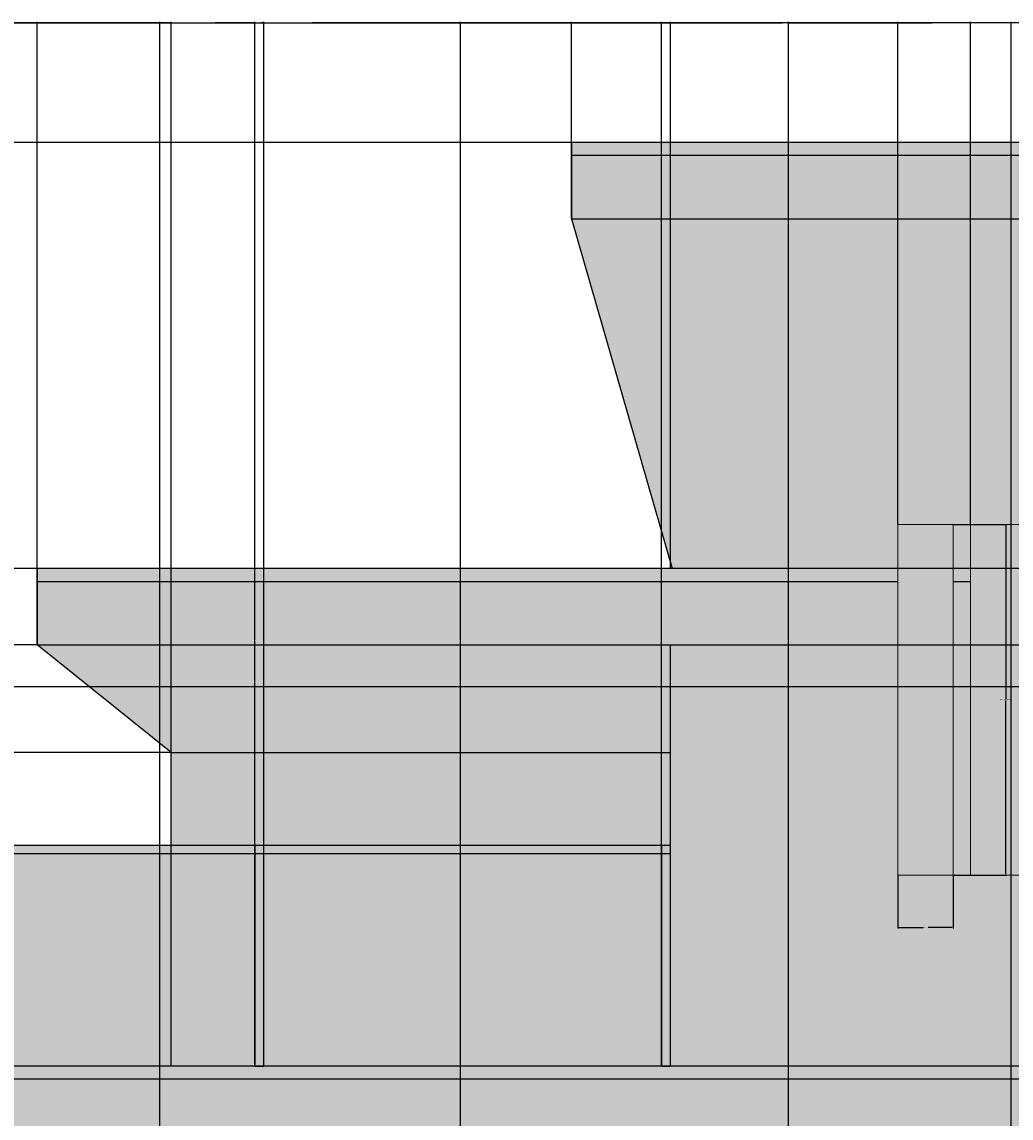
# Model space of a CAD drawing. Units: feet. Extents: x 2926 to 4178, y 965 to 1469.
# Tile 5 of 9: x 3040 to 3245, y 1241 to 1469. Entities that reach past the tile are written whole.
import ezdxf

# ---------------------------------------------------------------- set-up
doc = ezdxf.new("R2010")
doc.units = ezdxf.units.FT
for name, color, linetype, lineweight in [('A-ANNO-DIMS', 2, 'Continuous', 18), ('A-ELEV', 7, 'Continuous', 25), ('A-ELEV-DETL', 8, 'Continuous', 18), ('A-ELEV-PATT', 9, 'Continuous', 13)]:
    doc.layers.add(name, color=color, linetype=linetype, lineweight=lineweight)
doc.styles.get("Standard").update_dxf_attribs({"font": 'arial.ttf'})
doc.dimstyles.get("Standard").update_dxf_attribs({"dimtxt": 0.18, "dimasz": 0.18, "dimexe": 0.18, "dimexo": 0.0625, "dimgap": 0.09, "dimtad": 0, "dimtih": 1, "dimtoh": 1, "dimdec": 1, "dimzin": 0, "dimdsep": 46, "dimlunit": 3, "dimtxsty": 'Standard', "dimcen": 0.09, "dimadec": 0, "dimazin": 0, "dimtfac": 1, "dimtdec": 1, "dimtofl": 0, "dimtmove": 0, "dimatfit": 3, "dimfxl": 1, "dimtolj": 1, "dimtzin": 0, "dimarcsym": 0})

# ---------------------------------------------------------------- blocks, each defined once
blk = doc.blocks.new('FACADE-FIN')
blk.add_lwpolyline([(0, 72.66), (11.46, 72.66), (11.46, 0), (0, 0)], close=True)
blk.add_lwpolyline([(0, 72.66), (11.46, 72.66), (11.46, 0), (0, 0)], close=True)
blk = doc.blocks.new('*D4')
at = {"layer": 'A-ANNO-DIMS', "color": 0, "lineweight": -2, "transparency": 16777216}
for p, q in [((3232.87, 1364.4), (3243.89, 1364.4)), ((3243.71, 1364.22), (3243.71, 1328.25)), ((3243.71, 1291.91), (3243.71, 1327.88)), ((3232.87, 1291.73), (3243.89, 1291.73))]:
    blk.add_line(p, q, dxfattribs=at)
at = {"layer": 'A-ANNO-DIMS', "color": 0, "transparency": 16777216}
for points in [[(3243.68, 1364.22), (3243.74, 1364.22), (3243.71, 1364.4)], [(3243.68, 1291.91), (3243.74, 1291.91), (3243.71, 1291.73)]]:
    blk.add_solid(points, dxfattribs=at)
at = {"layer": 'Defpoints', "color": 0, "transparency": 16777216}
for p in [(3232.81, 1364.4), (3243.71, 1364.4), (3232.81, 1291.73)]:
    blk.add_point(p, dxfattribs=at)
at = {"layer": 'A-ANNO-DIMS', "color": 0, "transparency": 16777216, "insert": (3243.71, 1328.07), "char_height": 0.18, "attachment_point": 5}
blk.add_mtext('\\A1;FACADE FIN 73 TYP.', dxfattribs=at)
blk = doc.blocks.new('*D5')
at = {"layer": 'A-ANNO-DIMS', "color": 0, "lineweight": -2, "transparency": 16777216}
for p, q in [((3221.35, 1291.67), (3221.35, 1280.66)), ((3232.81, 1291.67), (3232.81, 1280.66)), ((3221.53, 1280.84), (3226.56, 1280.84)), ((3232.63, 1280.84), (3227.6, 1280.84))]:
    blk.add_line(p, q, dxfattribs=at)
at = {"layer": 'A-ANNO-DIMS', "color": 0, "transparency": 16777216}
for points in [[(3221.53, 1280.87), (3221.53, 1280.81), (3221.35, 1280.84)], [(3232.63, 1280.87), (3232.63, 1280.81), (3232.81, 1280.84)]]:
    blk.add_solid(points, dxfattribs=at)
at = {"layer": 'Defpoints', "color": 0, "transparency": 16777216}
for p in [(3221.35, 1291.73), (3232.81, 1291.73), (3232.81, 1280.84)]:
    blk.add_point(p, dxfattribs=at)
at = {"layer": 'A-ANNO-DIMS', "color": 0, "transparency": 16777216, "insert": (3227.08, 1280.84), "char_height": 0.18, "attachment_point": 5}
blk.add_mtext('\\A1;11 TYP.', dxfattribs=at)
blk = doc.blocks.new('*D10')
at = {"layer": 'A-ANNO-DIMS', "color": 0, "lineweight": -2, "transparency": 16777216}
for p, q in [((2952.4, 1298.4), (2952.4, 1468.62)), ((2952.58, 1468.44), (3195.09, 1468.44)), ((3438.39, 1468.44), (3195.88, 1468.44)), ((3438.57, 1443.71), (3438.57, 1468.62))]:
    blk.add_line(p, q, dxfattribs=at)
at = {"layer": 'A-ANNO-DIMS', "color": 0, "transparency": 16777216}
for points in [[(2952.58, 1468.47), (2952.58, 1468.41), (2952.4, 1468.44)], [(3438.39, 1468.47), (3438.39, 1468.41), (3438.57, 1468.44)]]:
    blk.add_solid(points, dxfattribs=at)
at = {"layer": 'Defpoints', "color": 0, "transparency": 16777216}
for p in [(3438.57, 1468.44), (3438.57, 1443.64), (2952.4, 1298.33)]:
    blk.add_point(p, dxfattribs=at)
at = {"layer": 'A-ANNO-DIMS', "color": 0, "transparency": 16777216, "insert": (3195.49, 1468.44), "char_height": 0.18, "attachment_point": 5}
blk.add_mtext('\\A1;486.2', dxfattribs=at)
blk = doc.blocks.new('*D17')
at = {"layer": 'A-ANNO-DIMS', "color": 0, "lineweight": -2, "transparency": 16777216}
for p, q in [((2952.34, 1252.14), (2926.57, 1252.14)), ((2926.75, 1251.96), (2926.75, 1235.86)), ((2926.75, 1219.4), (2926.75, 1235.5)), ((3198.58, 1219.22), (2926.57, 1219.22))]:
    blk.add_line(p, q, dxfattribs=at)
at = {"layer": 'A-ANNO-DIMS', "color": 0, "transparency": 16777216}
for points in [[(2926.72, 1251.96), (2926.78, 1251.96), (2926.75, 1252.14)], [(2926.72, 1219.4), (2926.78, 1219.4), (2926.75, 1219.22)]]:
    blk.add_solid(points, dxfattribs=at)
at = {"layer": 'Defpoints', "color": 0, "transparency": 16777216}
for p in [(2926.75, 1252.14), (2952.4, 1252.14), (3198.64, 1219.22)]:
    blk.add_point(p, dxfattribs=at)
at = {"layer": 'A-ANNO-DIMS', "color": 0, "transparency": 16777216, "insert": (2926.75, 1235.68), "char_height": 0.18, "attachment_point": 5}
blk.add_mtext('\\A1;32.92', dxfattribs=at)
blk = doc.blocks.new('*D19')
at = {"layer": 'A-ANNO-DIMS', "color": 0, "lineweight": -2, "transparency": 16777216}
for p, q in [((3335.85, 1330.74), (2926.57, 1330.74)), ((2926.75, 1330.56), (2926.75, 1314.5)), ((2926.75, 1298.08), (2926.75, 1314.14)), ((2952.34, 1297.9), (2926.57, 1297.9))]:
    blk.add_line(p, q, dxfattribs=at)
at = {"layer": 'A-ANNO-DIMS', "color": 0, "transparency": 16777216}
for points in [[(2926.72, 1330.56), (2926.78, 1330.56), (2926.75, 1330.74)], [(2926.72, 1298.08), (2926.78, 1298.08), (2926.75, 1297.9)]]:
    blk.add_solid(points, dxfattribs=at)
at = {"layer": 'Defpoints', "color": 0, "transparency": 16777216}
for p in [(2926.75, 1330.74), (3335.91, 1330.74), (2952.4, 1297.9)]:
    blk.add_point(p, dxfattribs=at)
at = {"layer": 'A-ANNO-DIMS', "color": 0, "transparency": 16777216, "insert": (2926.75, 1314.32), "char_height": 0.18, "attachment_point": 5}
blk.add_mtext('\\A1;32.85', dxfattribs=at)
blk = doc.blocks.new('*D20')
at = {"layer": 'A-ANNO-DIMS', "color": 0, "lineweight": -2, "transparency": 16777216}
for p, q in [((3042.86, 1355.28), (2926.57, 1355.28)), ((2926.75, 1355.1), (2926.75, 1343.19)), ((2926.75, 1330.92), (2926.75, 1342.83)), ((3335.85, 1330.74), (2926.57, 1330.74))]:
    blk.add_line(p, q, dxfattribs=at)
at = {"layer": 'A-ANNO-DIMS', "color": 0, "transparency": 16777216}
for points in [[(2926.72, 1355.1), (2926.78, 1355.1), (2926.75, 1355.28)], [(2926.72, 1330.92), (2926.78, 1330.92), (2926.75, 1330.74)]]:
    blk.add_solid(points, dxfattribs=at)
at = {"layer": 'Defpoints', "color": 0, "transparency": 16777216}
for p in [(2926.75, 1355.28), (3042.92, 1355.28), (3335.91, 1330.74)]:
    blk.add_point(p, dxfattribs=at)
at = {"layer": 'A-ANNO-DIMS', "color": 0, "transparency": 16777216, "insert": (2926.75, 1343.01), "char_height": 0.18, "attachment_point": 5}
blk.add_mtext('\\A1;24.533', dxfattribs=at)
blk = doc.blocks.new('*D21')
at = {"layer": 'A-ANNO-DIMS', "color": 0, "lineweight": -2, "transparency": 16777216}
for p, q in [((3153.63, 1443.64), (2926.57, 1443.64)), ((2926.75, 1443.46), (2926.75, 1399.64)), ((2926.75, 1355.46), (2926.75, 1399.28)), ((3042.86, 1355.28), (2926.57, 1355.28))]:
    blk.add_line(p, q, dxfattribs=at)
at = {"layer": 'A-ANNO-DIMS', "color": 0, "transparency": 16777216}
for points in [[(2926.72, 1443.46), (2926.78, 1443.46), (2926.75, 1443.64)], [(2926.72, 1355.46), (2926.78, 1355.46), (2926.75, 1355.28)]]:
    blk.add_solid(points, dxfattribs=at)
at = {"layer": 'Defpoints', "color": 0, "transparency": 16777216}
for p in [(2926.75, 1443.64), (3153.7, 1443.64), (3042.92, 1355.28)]:
    blk.add_point(p, dxfattribs=at)
at = {"layer": 'A-ANNO-DIMS', "color": 0, "transparency": 16777216, "insert": (2926.75, 1399.46), "char_height": 0.18, "attachment_point": 5}
blk.add_mtext('\\A1;88.37', dxfattribs=at)
blk = doc.blocks.new('*D22')
at = {"layer": 'A-ANNO-DIMS', "color": 0, "lineweight": -2, "transparency": 16777216}
for p, q in [((2952.4, 1056.38), (2952.4, 1468.62)), ((2952.58, 1468.44), (3009.97, 1468.44)), ((3068.13, 1468.44), (3010.74, 1468.44)), ((3068.31, 1050.05), (3068.31, 1468.62))]:
    blk.add_line(p, q, dxfattribs=at)
at = {"layer": 'A-ANNO-DIMS', "color": 0, "transparency": 16777216}
for points in [[(2952.58, 1468.47), (2952.58, 1468.41), (2952.4, 1468.44)], [(3068.13, 1468.47), (3068.13, 1468.41), (3068.31, 1468.44)]]:
    blk.add_solid(points, dxfattribs=at)
at = {"layer": 'Defpoints', "color": 0, "transparency": 16777216}
for p in [(3068.31, 1468.44), (2952.4, 1056.32), (3068.31, 1049.98)]:
    blk.add_point(p, dxfattribs=at)
at = {"layer": 'A-ANNO-DIMS', "color": 0, "transparency": 16777216, "insert": (3010.36, 1468.44), "char_height": 0.18, "attachment_point": 5}
blk.add_mtext('\\A1;115.9', dxfattribs=at)
blk = doc.blocks.new('*D23')
at = {"layer": 'A-ANNO-DIMS', "color": 0, "lineweight": -2, "transparency": 16777216}
for p, q in [((3068.31, 1050.05), (3068.31, 1468.62)), ((3068.49, 1468.44), (3099.11, 1468.44)), ((3130.51, 1468.44), (3099.9, 1468.44)), ((3130.69, 1050.05), (3130.69, 1468.62))]:
    blk.add_line(p, q, dxfattribs=at)
at = {"layer": 'A-ANNO-DIMS', "color": 0, "transparency": 16777216}
for points in [[(3068.49, 1468.47), (3068.49, 1468.41), (3068.31, 1468.44)], [(3130.51, 1468.47), (3130.51, 1468.41), (3130.69, 1468.44)]]:
    blk.add_solid(points, dxfattribs=at)
at = {"layer": 'Defpoints', "color": 0, "transparency": 16777216}
for p in [(3130.69, 1468.44), (3068.31, 1049.98), (3130.69, 1049.98)]:
    blk.add_point(p, dxfattribs=at)
at = {"layer": 'A-ANNO-DIMS', "color": 0, "transparency": 16777216, "insert": (3099.5, 1468.44), "char_height": 0.18, "attachment_point": 5}
blk.add_mtext('\\A1;62.38', dxfattribs=at)
blk = doc.blocks.new('*D24')
at = {"layer": 'A-ANNO-DIMS', "color": 0, "lineweight": -2, "transparency": 16777216}
for p, q in [((3130.69, 1050.05), (3130.69, 1468.62)), ((3130.87, 1468.44), (3164.27, 1468.44)), ((3198.46, 1468.44), (3165.06, 1468.44)), ((3198.64, 1133.35), (3198.64, 1468.62))]:
    blk.add_line(p, q, dxfattribs=at)
at = {"layer": 'A-ANNO-DIMS', "color": 0, "transparency": 16777216}
for points in [[(3130.87, 1468.47), (3130.87, 1468.41), (3130.69, 1468.44)], [(3198.46, 1468.47), (3198.46, 1468.41), (3198.64, 1468.44)]]:
    blk.add_solid(points, dxfattribs=at)
at = {"layer": 'Defpoints', "color": 0, "transparency": 16777216}
for p in [(3198.64, 1468.44), (3198.64, 1133.29), (3130.69, 1049.98)]:
    blk.add_point(p, dxfattribs=at)
at = {"layer": 'A-ANNO-DIMS', "color": 0, "transparency": 16777216, "insert": (3164.67, 1468.44), "char_height": 0.18, "attachment_point": 5}
blk.add_mtext('\\A1;67.95', dxfattribs=at)
blk = doc.blocks.new('*D25')
at = {"layer": 'A-ANNO-DIMS', "color": 0, "lineweight": -2, "transparency": 16777216}
for p, q in [((3198.64, 1133.35), (3198.64, 1468.62)), ((3198.82, 1468.44), (3221.33, 1468.44)), ((3244.64, 1468.44), (3222.13, 1468.44)), ((3244.82, 1133.35), (3244.82, 1468.62))]:
    blk.add_line(p, q, dxfattribs=at)
at = {"layer": 'A-ANNO-DIMS', "color": 0, "transparency": 16777216}
for points in [[(3198.82, 1468.47), (3198.82, 1468.41), (3198.64, 1468.44)], [(3244.64, 1468.47), (3244.64, 1468.41), (3244.82, 1468.44)]]:
    blk.add_solid(points, dxfattribs=at)
at = {"layer": 'Defpoints', "color": 0, "transparency": 16777216}
for p in [(3244.82, 1468.44), (3198.64, 1133.29), (3244.82, 1133.29)]:
    blk.add_point(p, dxfattribs=at)
at = {"layer": 'A-ANNO-DIMS', "color": 0, "transparency": 16777216, "insert": (3221.73, 1468.44), "char_height": 0.18, "attachment_point": 5}
blk.add_mtext('\\A1;46.18', dxfattribs=at)
blk = doc.blocks.new('*D29')
at = {"layer": 'A-ANNO-DIMS', "color": 0, "lineweight": -2, "transparency": 16777216}
for p, q in [((2952.4, 1298.4), (2952.4, 1468.62)), ((2952.58, 1468.44), (2997.27, 1468.44)), ((3042.74, 1468.44), (2998.05, 1468.44)), ((3042.92, 1355.34), (3042.92, 1468.62))]:
    blk.add_line(p, q, dxfattribs=at)
at = {"layer": 'A-ANNO-DIMS', "color": 0, "transparency": 16777216}
for points in [[(2952.58, 1468.47), (2952.58, 1468.41), (2952.4, 1468.44)], [(3042.74, 1468.47), (3042.74, 1468.41), (3042.92, 1468.44)]]:
    blk.add_solid(points, dxfattribs=at)
at = {"layer": 'Defpoints', "color": 0, "transparency": 16777216}
for p in [(3042.92, 1468.44), (3042.92, 1355.28), (2952.4, 1298.33)]:
    blk.add_point(p, dxfattribs=at)
at = {"layer": 'A-ANNO-DIMS', "color": 0, "transparency": 16777216, "insert": (2997.66, 1468.44), "char_height": 0.18, "attachment_point": 5}
blk.add_mtext('\\A1;90.52', dxfattribs=at)
blk = doc.blocks.new('*D30')
at = {"layer": 'A-ANNO-DIMS', "color": 0, "lineweight": -2, "transparency": 16777216}
for p, q in [((3042.92, 1339.53), (3042.92, 1468.62)), ((3043.1, 1468.44), (3056.41, 1468.44)), ((3070.5, 1468.44), (3057.2, 1468.44)), ((3070.68, 1317.25), (3070.68, 1468.62))]:
    blk.add_line(p, q, dxfattribs=at)
at = {"layer": 'A-ANNO-DIMS', "color": 0, "transparency": 16777216}
for points in [[(3043.1, 1468.47), (3043.1, 1468.41), (3042.92, 1468.44)], [(3070.5, 1468.47), (3070.5, 1468.41), (3070.68, 1468.44)]]:
    blk.add_solid(points, dxfattribs=at)
at = {"layer": 'Defpoints', "color": 0, "transparency": 16777216}
for p in [(3070.68, 1468.44), (3042.92, 1339.46), (3070.68, 1317.18)]:
    blk.add_point(p, dxfattribs=at)
at = {"layer": 'A-ANNO-DIMS', "color": 0, "transparency": 16777216, "insert": (3056.8, 1468.44), "char_height": 0.18, "attachment_point": 5}
blk.add_mtext('\\A1;27.76', dxfattribs=at)
blk = doc.blocks.new('*D31')
at = {"layer": 'A-ANNO-DIMS', "color": 0, "lineweight": -2, "transparency": 16777216}
for p, q in [((3070.68, 1317.25), (3070.68, 1468.62)), ((3070.86, 1468.44), (3111.81, 1468.44)), ((3153.52, 1468.44), (3112.56, 1468.44)), ((3153.7, 1427.89), (3153.7, 1468.62))]:
    blk.add_line(p, q, dxfattribs=at)
at = {"layer": 'A-ANNO-DIMS', "color": 0, "transparency": 16777216}
for points in [[(3070.86, 1468.47), (3070.86, 1468.41), (3070.68, 1468.44)], [(3153.52, 1468.47), (3153.52, 1468.41), (3153.7, 1468.44)]]:
    blk.add_solid(points, dxfattribs=at)
at = {"layer": 'Defpoints', "color": 0, "transparency": 16777216}
for p in [(3153.7, 1468.44), (3153.7, 1427.83), (3070.68, 1317.18)]:
    blk.add_point(p, dxfattribs=at)
at = {"layer": 'A-ANNO-DIMS', "color": 0, "transparency": 16777216, "insert": (3112.19, 1468.44), "char_height": 0.18, "attachment_point": 5}
blk.add_mtext('\\A1;83.01', dxfattribs=at)
blk = doc.blocks.new('*D32')
at = {"layer": 'A-ANNO-DIMS', "color": 0, "lineweight": -2, "transparency": 16777216}
for p, q in [((3153.7, 1427.89), (3153.7, 1468.62)), ((3153.88, 1468.44), (3163.56, 1468.44)), ((3174.04, 1468.44), (3164.35, 1468.44)), ((3174.22, 1355.34), (3174.22, 1468.62))]:
    blk.add_line(p, q, dxfattribs=at)
at = {"layer": 'A-ANNO-DIMS', "color": 0, "transparency": 16777216}
for points in [[(3153.88, 1468.47), (3153.88, 1468.41), (3153.7, 1468.44)], [(3174.04, 1468.47), (3174.04, 1468.41), (3174.22, 1468.44)]]:
    blk.add_solid(points, dxfattribs=at)
at = {"layer": 'Defpoints', "color": 0, "transparency": 16777216}
for p in [(3174.22, 1468.44), (3153.7, 1427.83), (3174.22, 1355.28)]:
    blk.add_point(p, dxfattribs=at)
at = {"layer": 'A-ANNO-DIMS', "color": 0, "transparency": 16777216, "insert": (3163.96, 1468.44), "char_height": 0.18, "attachment_point": 5}
blk.add_mtext('\\A1;20.52', dxfattribs=at)
blk = doc.blocks.new('*D33')
at = {"layer": 'A-ANNO-DIMS', "color": 0, "lineweight": -2, "transparency": 16777216}
for p, q in [((3174.22, 1355.34), (3174.22, 1468.62)), ((3174.4, 1468.44), (3197.39, 1468.44)), ((3221.17, 1468.44), (3198.18, 1468.44)), ((3221.35, 1364.46), (3221.35, 1468.62))]:
    blk.add_line(p, q, dxfattribs=at)
at = {"layer": 'A-ANNO-DIMS', "color": 0, "transparency": 16777216}
for points in [[(3174.4, 1468.47), (3174.4, 1468.41), (3174.22, 1468.44)], [(3221.17, 1468.47), (3221.17, 1468.41), (3221.35, 1468.44)]]:
    blk.add_solid(points, dxfattribs=at)
at = {"layer": 'Defpoints', "color": 0, "transparency": 16777216}
for p in [(3221.35, 1468.44), (3221.35, 1364.4), (3174.22, 1355.28)]:
    blk.add_point(p, dxfattribs=at)
at = {"layer": 'A-ANNO-DIMS', "color": 0, "transparency": 16777216, "insert": (3197.78, 1468.44), "char_height": 0.18, "attachment_point": 5}
blk.add_mtext('\\A1;47.13', dxfattribs=at)
blk = doc.blocks.new('*D34')
at = {"layer": 'A-ANNO-DIMS', "color": 0, "lineweight": -2, "transparency": 16777216}
for p, q in [((3221.35, 1364.46), (3221.35, 1468.62)), ((3221.53, 1468.44), (3228.49, 1468.44)), ((3236.23, 1468.44), (3229.26, 1468.44)), ((3236.41, 1364.46), (3236.41, 1468.62))]:
    blk.add_line(p, q, dxfattribs=at)
at = {"layer": 'A-ANNO-DIMS', "color": 0, "transparency": 16777216}
for points in [[(3221.53, 1468.47), (3221.53, 1468.41), (3221.35, 1468.44)], [(3236.23, 1468.47), (3236.23, 1468.41), (3236.41, 1468.44)]]:
    blk.add_solid(points, dxfattribs=at)
at = {"layer": 'Defpoints', "color": 0, "transparency": 16777216}
for p in [(3236.41, 1468.44), (3221.35, 1364.4), (3236.41, 1364.4)]:
    blk.add_point(p, dxfattribs=at)
at = {"layer": 'A-ANNO-DIMS', "color": 0, "transparency": 16777216, "insert": (3228.88, 1468.44), "char_height": 0.18, "attachment_point": 5}
blk.add_mtext('\\A1;15.06', dxfattribs=at)
blk = doc.blocks.new('*D41')
at = {"layer": 'A-ANNO-DIMS', "color": 0, "lineweight": -2, "transparency": 16777216}
for p, q in [((3042.86, 1355.28), (2926.57, 1355.28)), ((2926.75, 1355.1), (2926.75, 1347.55)), ((2926.75, 1339.64), (2926.75, 1347.19)), ((3042.86, 1339.46), (2926.57, 1339.46))]:
    blk.add_line(p, q, dxfattribs=at)
at = {"layer": 'A-ANNO-DIMS', "color": 0, "transparency": 16777216}
for points in [[(2926.72, 1355.1), (2926.78, 1355.1), (2926.75, 1355.28)], [(2926.72, 1339.64), (2926.78, 1339.64), (2926.75, 1339.46)]]:
    blk.add_solid(points, dxfattribs=at)
at = {"layer": 'Defpoints', "color": 0, "transparency": 16777216}
for p in [(2926.75, 1355.28), (3042.92, 1355.28), (3042.92, 1339.46)]:
    blk.add_point(p, dxfattribs=at)
at = {"layer": 'A-ANNO-DIMS', "color": 0, "transparency": 16777216, "insert": (2926.75, 1347.37), "char_height": 0.18, "attachment_point": 5}
blk.add_mtext('\\A1;15.814', dxfattribs=at)
blk = doc.blocks.new('*D42')
at = {"layer": 'A-ANNO-DIMS', "color": 0, "lineweight": -2, "transparency": 16777216}
for p, q in [((3042.86, 1339.46), (2926.57, 1339.46)), ((2926.75, 1339.28), (2926.75, 1328.51)), ((2926.75, 1317.36), (2926.75, 1328.14)), ((3070.62, 1317.18), (2926.57, 1317.18))]:
    blk.add_line(p, q, dxfattribs=at)
at = {"layer": 'A-ANNO-DIMS', "color": 0, "transparency": 16777216}
for points in [[(2926.72, 1339.28), (2926.78, 1339.28), (2926.75, 1339.46)], [(2926.72, 1317.36), (2926.78, 1317.36), (2926.75, 1317.18)]]:
    blk.add_solid(points, dxfattribs=at)
at = {"layer": 'Defpoints', "color": 0, "transparency": 16777216}
for p in [(2926.75, 1339.46), (3042.92, 1339.46), (3070.68, 1317.18)]:
    blk.add_point(p, dxfattribs=at)
at = {"layer": 'A-ANNO-DIMS', "color": 0, "transparency": 16777216, "insert": (2926.75, 1328.32), "char_height": 0.18, "attachment_point": 5}
blk.add_mtext('\\A1;22.28', dxfattribs=at)
blk = doc.blocks.new('*D46')
at = {"layer": 'A-ANNO-DIMS', "color": 0, "lineweight": -2, "transparency": 16777216}
for p, q in [((3006.65, 1252.2), (3006.65, 1468.62)), ((3006.83, 1468.44), (3038.27, 1468.44)), ((3070.5, 1468.44), (3039.06, 1468.44)), ((3070.68, 1317.25), (3070.68, 1468.62))]:
    blk.add_line(p, q, dxfattribs=at)
at = {"layer": 'A-ANNO-DIMS', "color": 0, "transparency": 16777216}
for points in [[(3006.83, 1468.47), (3006.83, 1468.41), (3006.65, 1468.44)], [(3070.5, 1468.47), (3070.5, 1468.41), (3070.68, 1468.44)]]:
    blk.add_solid(points, dxfattribs=at)
at = {"layer": 'Defpoints', "color": 0, "transparency": 16777216}
for p in [(3070.68, 1468.44), (3070.68, 1317.18), (3006.65, 1252.14)]:
    blk.add_point(p, dxfattribs=at)
at = {"layer": 'A-ANNO-DIMS', "color": 0, "transparency": 16777216, "insert": (3038.66, 1468.44), "char_height": 0.18, "attachment_point": 5}
blk.add_mtext('\\A1;64.03', dxfattribs=at)
blk = doc.blocks.new('*D47')
at = {"layer": 'A-ANNO-DIMS', "color": 0, "lineweight": -2, "transparency": 16777216}
for p, q in [((3070.68, 1252.2), (3070.68, 1468.62)), ((3070.86, 1468.44), (3078.88, 1468.44)), ((3087.82, 1468.44), (3079.79, 1468.44)), ((3088, 1252.2), (3088, 1468.62))]:
    blk.add_line(p, q, dxfattribs=at)
at = {"layer": 'A-ANNO-DIMS', "color": 0, "transparency": 16777216}
for points in [[(3070.86, 1468.47), (3070.86, 1468.41), (3070.68, 1468.44)], [(3087.82, 1468.47), (3087.82, 1468.41), (3088, 1468.44)]]:
    blk.add_solid(points, dxfattribs=at)
at = {"layer": 'Defpoints', "color": 0, "transparency": 16777216}
for p in [(3088, 1468.44), (3070.68, 1252.14), (3088, 1252.14)]:
    blk.add_point(p, dxfattribs=at)
at = {"layer": 'A-ANNO-DIMS', "color": 0, "transparency": 16777216, "insert": (3079.34, 1468.44), "char_height": 0.18, "attachment_point": 5}
blk.add_mtext('\\A1;17.316', dxfattribs=at)
blk = doc.blocks.new('*D48')
at = {"layer": 'A-ANNO-DIMS', "color": 0, "lineweight": -2, "transparency": 16777216}
for p, q in [((3088, 1297.96), (3088, 1468.62)), ((3088.18, 1468.44), (3088.62, 1468.44)), ((3089.69, 1468.44), (3089.25, 1468.44)), ((3089.87, 1297.96), (3089.87, 1468.62))]:
    blk.add_line(p, q, dxfattribs=at)
at = {"layer": 'A-ANNO-DIMS', "color": 0, "transparency": 16777216}
for points in [[(3088.18, 1468.47), (3088.18, 1468.41), (3088, 1468.44)], [(3089.69, 1468.47), (3089.69, 1468.41), (3089.87, 1468.44)]]:
    blk.add_solid(points, dxfattribs=at)
at = {"layer": 'Defpoints', "color": 0, "transparency": 16777216}
for p in [(3089.87, 1468.44), (3088, 1297.9), (3089.87, 1297.9)]:
    blk.add_point(p, dxfattribs=at)
at = {"layer": 'A-ANNO-DIMS', "color": 0, "transparency": 16777216, "insert": (3088.93, 1468.44), "char_height": 0.18, "attachment_point": 5}
blk.add_mtext('\\A1;1.87', dxfattribs=at)
blk = doc.blocks.new('*D49')
at = {"layer": 'A-ANNO-DIMS', "color": 0, "lineweight": -2, "transparency": 16777216}
for p, q in [((3089.87, 1252.2), (3089.87, 1468.62)), ((3090.05, 1468.44), (3130.71, 1468.44)), ((3172.17, 1468.44), (3131.5, 1468.44)), ((3172.35, 1252.2), (3172.35, 1468.62))]:
    blk.add_line(p, q, dxfattribs=at)
at = {"layer": 'A-ANNO-DIMS', "color": 0, "transparency": 16777216}
for points in [[(3090.05, 1468.47), (3090.05, 1468.41), (3089.87, 1468.44)], [(3172.17, 1468.47), (3172.17, 1468.41), (3172.35, 1468.44)]]:
    blk.add_solid(points, dxfattribs=at)
at = {"layer": 'Defpoints', "color": 0, "transparency": 16777216}
for p in [(3172.35, 1468.44), (3089.87, 1252.14), (3172.35, 1252.14)]:
    blk.add_point(p, dxfattribs=at)
at = {"layer": 'A-ANNO-DIMS', "color": 0, "transparency": 16777216, "insert": (3131.11, 1468.44), "char_height": 0.18, "attachment_point": 5}
blk.add_mtext('\\A1;82.48', dxfattribs=at)

msp = doc.modelspace()

# ---------------------------------------------------------------- hatches: boundary and pattern name
at = {"layer": 'A-ELEV-PATT'}
h = msp.add_hatch(color=256, dxfattribs=at)
h.dxf.hatch_style = 1
h.paths.add_polyline_path([(2968.9852, 1110.3246), (2958.1139, 1110.3246), (2958.1139, 1060.462), (2968.9852, 1060.462)])
h.paths.add_polyline_path([(3174.217, 1126.1389), (2952.4018, 1126.1389), (2952.4018, 1110.3246), (3174.217, 1110.3246), (3273.5987, 1110.3246), (3273.5987, 1116.3246), (3174.217, 1116.3246)], flags=17)
h.paths.add_polyline_path([(3289.413, 1252.1389), (2952.4018, 1252.1389), (2952.4018, 1236.3246), (3273.5987, 1236.3246), (3273.5987, 1110.3246), (3289.413, 1110.3246)])
h.paths.add_polyline_path([(3221.3497, 1355.2778), (3042.9199, 1355.2778), (3042.9199, 1339.4635), (3221.3497, 1339.4635)])
h.paths.add_polyline_path([(3379.9311, 1355.2778), (3262.1646, 1355.2778), (3262.1646, 1339.4635), (3364.1168, 1339.4635), (3364.1168, 990.3246), (3379.9311, 990.3246)])
h.paths.add_polyline_path([(3364.1168, 1330.7444), (3335.9143, 1330.7444), (3335.9143, 1023.8561), (3364.1168, 1023.8561), (3364.1168, 1027.6935), (3339.7517, 1027.6935), (3339.7517, 1326.907), (3364.1168, 1326.907)], flags=17)
h.paths.add_polyline_path([(3438.5707, 1443.6445), (3153.6951, 1443.6445), (3153.6951, 1427.8302), (3438.5707, 1427.8302)])
h.paths.add_polyline_path([(3174.217, 1427.8302), (3153.6951, 1427.8302), (3174.217, 1356.4366)])
h.paths.add_polyline_path([(3174.217, 1339.4635), (3042.9199, 1339.4635), (3070.6809, 1317.1829), (3174.217, 1317.1829)])
h.paths.add_polyline_path([(3244.819, 1219.2195), (3198.6415, 1219.2195), (3198.6415, 1133.2879), (3244.819, 1133.2879)], flags=17)
h = msp.add_hatch(color=256, dxfattribs=at)
h.dxf.hatch_style = 1
h.paths.add_polyline_path([(3006.649, 1296.2176), (2952.4018, 1296.2176), (2952.4018, 1252.1389), (3006.649, 1252.1389)])
h.paths.add_polyline_path([(3084.0314, 1226.8042), (3008.2802, 1226.8042), (3008.2802, 1171.8963), (3084.0314, 1171.8963)])
h.paths.add_polyline_path([(3004.9276, 1228.4641), (2995.6704, 1228.4641), (2995.6704, 1171.8963), (3004.9276, 1171.8963)])
h.paths.add_polyline_path([(3174.217, 1236.3246), (3084.0314, 1236.3246), (3084.0314, 1171.8963), (3124.7575, 1171.8963), (3124.7575, 1207.1083), (3154.7729, 1207.1083), (3154.7729, 1171.8963), (3174.217, 1171.8963)])
h.paths.add_polyline_path([(3273.5987, 1236.3246), (3174.217, 1236.3246), (3174.217, 1171.8963), (3174.217, 1126.1389), (3174.217, 1116.3246), (3273.5987, 1116.3246)], flags=16)
h.paths.add_polyline_path([(3198.6415, 1219.2195), (3244.819, 1219.2195), (3244.819, 1133.2879), (3198.6415, 1133.2879)], flags=0)
h.paths.add_polyline_path([(3432.4018, 1427.8302), (3174.217, 1427.8302), (3174.217, 1356.4366), (3174.5501, 1355.2778), (3221.3497, 1355.2778), (3221.3497, 1364.3965), (3232.8063, 1364.3965), (3232.8063, 1355.2778), (3236.4098, 1355.2778), (3236.4098, 1364.3965), (3247.8663, 1364.3965), (3247.8663, 1355.2778), (3250.7081, 1355.2778), (3250.7081, 1364.3965), (3262.1646, 1364.3965), (3262.1646, 1355.2778), (3379.9311, 1355.2778), (3379.9311, 990.3246), (3432.4018, 990.3246)])
h.paths.add_polyline_path([(3068.3128, 1092.0439), (3130.6886, 1092.0439), (3130.6886, 1049.9841), (3146.6469, 1049.9841), (3146.6469, 1057.7915), (3145.2184, 1058.2122), (3145.2184, 1060.462), (3168.644, 1060.462), (3174.217, 1058.8204), (3174.217, 1110.3246), (3004.9276, 1110.3246), (3004.9276, 1049.9841), (3068.3128, 1049.9841)])
h.paths.add_polyline_path([(3174.217, 1056.3197), (3152.4954, 1056.3197), (3152.4954, 990.3246), (3174.217, 990.3246)])
h.paths.add_polyline_path([(2974.1234, 1056.3197), (2952.4018, 1056.3197), (2952.4018, 990.3246), (2974.1234, 990.3246)])
h.paths.add_polyline_path([(3004.9276, 1110.3246), (2995.6704, 1110.3246), (2995.6704, 1049.9841), (3004.9276, 1049.9841)])
h = msp.add_hatch(color=256, dxfattribs=at)
h.dxf.hatch_style = 1
h.paths.add_polyline_path([(3262.1646, 1339.4635), (3250.7081, 1339.4635), (3250.7081, 1291.7348), (3262.1646, 1291.7348)])
h.paths.add_polyline_path([(3262.1646, 1355.2778), (3250.7081, 1355.2778), (3250.7081, 1339.4635), (3262.1646, 1339.4635)])
h.paths.add_polyline_path([(3262.1646, 1364.3965), (3250.7081, 1364.3965), (3250.7081, 1355.2778), (3262.1646, 1355.2778)])
h.paths.add_polyline_path([(3247.8663, 1364.3965), (3236.4098, 1364.3965), (3236.4098, 1355.2778), (3247.8663, 1355.2778)])
h.paths.add_polyline_path([(3247.8663, 1355.2778), (3236.4098, 1355.2778), (3236.4098, 1339.4635), (3247.8663, 1339.4635)])
h.paths.add_polyline_path([(3247.8663, 1339.4635), (3236.4098, 1339.4635), (3236.4098, 1291.7348), (3247.8663, 1291.7348)])
h.paths.add_polyline_path([(3232.8063, 1339.4635), (3221.3497, 1339.4635), (3221.3497, 1291.7348), (3232.8063, 1291.7348)])
h.paths.add_polyline_path([(3232.8063, 1355.2778), (3221.3497, 1355.2778), (3221.3497, 1339.4635), (3232.8063, 1339.4635)])
h.paths.add_polyline_path([(3232.8063, 1364.3965), (3221.3497, 1364.3965), (3221.3497, 1355.2778), (3232.8063, 1355.2778)])
h = msp.add_hatch(color=256, dxfattribs=at)
h.dxf.hatch_style = 1
h.paths.add_polyline_path([(3335.9143, 1330.7444), (3364.1168, 1330.7444), (3364.1168, 1339.4635), (3262.1646, 1339.4635), (3262.1646, 1291.7348), (3250.7081, 1291.7348), (3250.7081, 1339.4635), (3247.8663, 1339.4635), (3247.8663, 1291.7348), (3236.4098, 1291.7348), (3236.4098, 1339.4635), (3232.8063, 1339.4635), (3232.8063, 1291.7348), (3221.3497, 1291.7348), (3221.3497, 1339.4635), (3174.217, 1339.4635), (3174.217, 1252.1389), (3289.413, 1252.1389), (3289.413, 1236.3246), (3289.413, 1110.3246), (3289.413, 1038.9216), (3174.217, 1038.9216), (3174.217, 990.3246), (3364.1168, 990.3246), (3364.1168, 1023.8561), (3335.9143, 1023.8561)])
h.paths.add_polyline_path([(3236.4098, 1355.2778), (3232.8063, 1355.2778), (3232.8063, 1339.4635), (3236.4098, 1339.4635)])
h.paths.add_polyline_path([(3250.7081, 1355.2778), (3247.8663, 1355.2778), (3247.8663, 1339.4635), (3250.7081, 1339.4635)])
h = msp.add_hatch(color=256, dxfattribs=at)
h.dxf.hatch_style = 1
h.paths.add_polyline_path([(3174.217, 1297.8963), (3172.3488, 1297.8963), (3006.649, 1297.8963), (3006.649, 1296.2176), (3087.9974, 1296.2176), (3087.9974, 1252.1389), (3089.8656, 1252.1389), (3089.8656, 1296.2176), (3172.3488, 1296.2176), (3172.3488, 1252.1389), (3174.217, 1252.1389)])
h.paths.add_polyline_path([(3102.4583, 1170.2176), (3172.3488, 1170.2176), (3172.3488, 1126.1389), (3174.217, 1126.1389), (3174.217, 1171.8963), (3172.3488, 1171.8963), (2952.4018, 1171.8963), (2952.4018, 1170.2176), (2952.4018, 1126.1389), (2954.27, 1126.1389), (2954.27, 1170.2176), (3100.5901, 1170.2176), (3100.5901, 1126.1389), (3102.4583, 1126.1389)])
h.paths.add_polyline_path([(3130.6886, 1092.0439), (3068.3128, 1092.0439), (3068.3128, 1049.9841), (3130.6886, 1049.9841)])
h.paths.add_polyline_path([(3099.0016, 1090.4638), (3099.0016, 1051.5643), (3069.893, 1051.5643), (3069.893, 1090.4638)], flags=16)
h.paths.add_polyline_path([(3099.9998, 1090.4638), (3129.1085, 1090.4638), (3129.1085, 1051.5643), (3099.9998, 1051.5643)], flags=16)
h.paths.add_polyline_path([(3067.2712, 1049.9841), (3060.102, 1049.9841), (3060.102, 990.3246), (3067.2712, 990.3246)])
h.paths.add_polyline_path([(3339.7517, 1326.907), (3364.1168, 1326.907), (3364.1168, 1330.7444), (3335.9143, 1330.7444), (3335.9143, 1023.8561), (3364.1168, 1023.8561), (3364.1168, 1027.6935), (3339.7517, 1027.6935)])
h.paths.add_polyline_path([(3154.7729, 1207.1083), (3124.7575, 1207.1083), (3124.7575, 1171.8963), (3126.8684, 1171.8963), (3126.8684, 1204.9974), (3152.6619, 1204.9974), (3152.6619, 1171.8963), (3154.7729, 1171.8963)])
h = msp.add_hatch(color=256, dxfattribs=at)
h.dxf.hatch_style = 1
h.paths.add_polyline_path([(3070.6809, 1296.2176), (3006.649, 1296.2176), (3006.649, 1252.1389), (3070.6809, 1252.1389)])
h.paths.add_polyline_path([(3087.9974, 1296.2176), (3070.6809, 1296.2176), (3070.6809, 1252.1389), (3087.9974, 1252.1389)])
h.paths.add_polyline_path([(3172.3488, 1296.2176), (3089.8656, 1296.2176), (3089.8656, 1252.1389), (3172.3488, 1252.1389)])
h.paths.add_polyline_path([(3152.6619, 1170.2176), (3126.8684, 1170.2176), (3126.8684, 1128.2498), (3152.6619, 1128.2498)], flags=17)
h.paths.add_polyline_path([(3152.6619, 1204.9974), (3126.8684, 1204.9974), (3126.8684, 1171.8963), (3152.6619, 1171.8963)])
h.paths.add_polyline_path([(3172.3488, 1170.2176), (3154.7729, 1170.2176), (3154.7729, 1126.1389), (3172.3488, 1126.1389)])
h.paths.add_polyline_path([(3154.7729, 1170.2176), (3152.6619, 1170.2176), (3152.6619, 1128.2498), (3126.8684, 1128.2498), (3126.8684, 1170.2176), (3124.7575, 1170.2176), (3124.7575, 1126.1389), (3154.7729, 1126.1389)])
h.paths.add_polyline_path([(3124.7575, 1170.2176), (3102.4583, 1170.2176), (3102.4583, 1126.1389), (3124.7575, 1126.1389)])
h.paths.add_polyline_path([(3100.5901, 1170.2176), (3084.0314, 1170.2176), (3084.0314, 1126.1389), (3100.5901, 1126.1389)])
h.paths.add_polyline_path([(3084.0314, 1170.2176), (3008.2802, 1170.2176), (3008.2802, 1126.1389), (3084.0314, 1126.1389)])
h.paths.add_polyline_path([(2995.6704, 1170.2176), (2971.1978, 1170.2176), (2971.1978, 1126.1389), (2995.6704, 1126.1389)])
h.paths.add_polyline_path([(3004.9276, 1170.2176), (2995.6704, 1170.2176), (2995.6704, 1126.1389), (3004.9276, 1126.1389)])
h.paths.add_polyline_path([(3364.1168, 1326.907), (3339.7517, 1326.907), (3339.7517, 1027.6935), (3364.1168, 1027.6935)])
h.paths.add_polyline_path([(3099.0016, 1090.4638), (3069.893, 1090.4638), (3069.893, 1051.5643), (3099.0016, 1051.5643)])
h.paths.add_polyline_path([(3129.1085, 1090.4638), (3099.9998, 1090.4638), (3099.9998, 1051.5643), (3129.1085, 1051.5643)])
h.paths.add_polyline_path([(2968.9852, 1170.2176), (2958.1139, 1170.2176), (2958.1139, 1126.1389), (2968.9852, 1126.1389)])
h.paths.add_polyline_path([(2958.1139, 1170.2176), (2954.27, 1170.2176), (2954.27, 1126.1389), (2958.1139, 1126.1389)])
h.paths.add_polyline_path([(2971.1978, 1170.2176), (2968.9852, 1170.2176), (2968.9852, 1126.1389), (2971.1978, 1126.1389)])
h = msp.add_hatch(color=256, dxfattribs=at)
h.dxf.hatch_style = 1
h.paths.add_polyline_path([(3174.217, 1317.1829), (3070.6809, 1317.1829), (3070.6809, 1297.8963), (3174.217, 1297.8963)])

# ---------------------------------------------------------------- linework, layer by layer
at = {"layer": 'A-ELEV'}
for p, q in [((3153.6951, 1440.9727), (3438.5707, 1440.9727)), ((3153.6951, 1427.8302), (3174.5501, 1355.2778)), ((3153.6951, 1427.8302), (3174.5501, 1355.2778)), ((3174.217, 1355.2778), (3174.217, 1427.8302)), ((3174.217, 1355.2778), (3174.217, 1427.8302)), ((3042.9199, 1352.606), (3221.3497, 1352.606)), ((3232.8063, 1352.606), (3236.4098, 1352.606)), ((3070.6809, 1317.1829), (3042.9199, 1339.4635)), ((3042.9199, 1339.4635), (3174.217, 1339.4635)), ((3070.6809, 1317.1829), (3042.9199, 1339.4635)), ((3042.9199, 1339.4635), (3174.217, 1339.4635)), ((3174.217, 1252.1389), (3174.217, 1339.4635)), ((3174.217, 1252.1389), (3174.217, 1339.4635)), ((3070.6809, 1252.1389), (3070.6809, 1317.1829)), ((3070.6809, 1317.1829), (3174.217, 1317.1829)), ((3070.6809, 1252.1389), (3070.6809, 1317.1829)), ((3070.6809, 1317.1829), (3174.217, 1317.1829)), ((2952.4018, 1249.4671), (3289.413, 1249.4671))]:
    msp.add_line(p, q, dxfattribs=at)
for points in [[(3438.5707, 1443.6445), (3153.6951, 1443.6445), (3153.6951, 1427.8302), (3438.5707, 1427.8302)], [(3438.5707, 1443.6445), (3153.6951, 1443.6445), (3153.6951, 1427.8302), (3438.5707, 1427.8302)], [(3379.9311, 990.3246), (3379.9311, 1355.2778), (3042.9199, 1355.2778), (3042.9199, 1339.4635), (3364.1168, 1339.4635)], [(3221.3497, 1355.2778), (3042.9199, 1355.2778), (3042.9199, 1339.4635), (3221.3497, 1339.4635)], [(3236.4098, 1355.2778), (3232.8063, 1355.2778)], [(3232.8063, 1339.4635), (3236.4098, 1339.4635)], [(2952.4018, 1297.8963), (2952.4018, 1296.2176), (3174.217, 1296.2176), (3174.217, 1297.8963), (3006.649, 1297.8963)], [(2952.4018, 1297.8963), (2952.4018, 1296.2176), (3174.217, 1296.2176), (3174.217, 1297.8963), (3006.649, 1297.8963)], [(3289.413, 1236.3246), (3289.413, 1252.1389), (2952.4018, 1252.1389), (2952.4018, 1236.3246), (3273.5987, 1236.3246)], [(3289.413, 1236.3246), (3289.413, 1252.1389), (2952.4018, 1252.1389), (2952.4018, 1236.3246), (3273.5987, 1236.3246)]]:
    msp.add_lwpolyline(points, dxfattribs=at)
for points in [[(3087.9974, 1252.1389), (3089.8656, 1252.1389), (3089.8656, 1297.8963), (3087.9974, 1297.8963)], [(3087.9974, 1252.1389), (3089.8656, 1252.1389), (3089.8656, 1297.8963), (3087.9974, 1297.8963)], [(3172.3488, 1252.1389), (3174.217, 1252.1389), (3174.217, 1297.8963), (3172.3488, 1297.8963)], [(3172.3488, 1252.1389), (3174.217, 1252.1389), (3174.217, 1297.8963), (3172.3488, 1297.8963)]]:
    msp.add_lwpolyline(points, close=True, dxfattribs=at)

# ---------------------------------------------------------------- block references
at = {"layer": 'A-ELEV-DETL'}
for p in [(3221.35, 1291.735), (3236.4101, 1291.735)]:
    msp.add_blockref('FACADE-FIN', p, dxfattribs=at)

# ---------------------------------------------------------------- dimensions: what is measured, and where the dimension line sits
at = {"layer": 'A-ANNO-DIMS'}
for base, p1, p2, override, picture, middle in [((3438.5707, 1468.4445), (2952.4018, 1298.3338), (3438.5707, 1443.6445), {"dimdec": 1, "dimlfac": 1, "dimrnd": 0, "dimzin": 0, "dimdsep": 46, "dimlunit": 2}, '*D10', (3195.4862, 1468.4445)), ((3068.3128, 1468.4445), (2952.4018, 1056.3197), (3068.3128, 1049.9841), {"dimdec": 1, "dimlfac": 1, "dimrnd": 0, "dimzin": 0, "dimdsep": 46, "dimlunit": 2}, '*D22', (3010.3573, 1468.4445)), ((3042.9199, 1468.4445), (2952.4018, 1298.3338), (3042.9199, 1355.2778), {"dimdec": 2, "dimlfac": 1, "dimrnd": 0, "dimzin": 0, "dimdsep": 46, "dimlunit": 2}, '*D29', (2997.6609, 1468.4445)), ((3070.6809, 1468.4445), (3006.649, 1252.1389), (3070.6809, 1317.1829), {"dimdec": 2, "dimlfac": 1, "dimrnd": 0, "dimzin": 0, "dimdsep": 46, "dimlunit": 2}, '*D46', (3038.665, 1468.4445)), ((3070.6809, 1468.4445), (3042.9199, 1339.4635), (3070.6809, 1317.1829), {"dimdec": 2, "dimlfac": 1, "dimrnd": 0, "dimzin": 0, "dimdsep": 46, "dimlunit": 2}, '*D30', (3056.8004, 1468.4445)), ((3130.6886, 1468.4445), (3068.3128, 1049.9841), (3130.6886, 1049.9841), {"dimdec": 2, "dimlfac": 1, "dimrnd": 0, "dimzin": 0, "dimdsep": 46, "dimlunit": 2}, '*D23', (3099.5007, 1468.4445)), ((3153.6951, 1468.4445), (3070.6809, 1317.1829), (3153.6951, 1427.8302), {"dimdec": 2, "dimlfac": 1, "dimrnd": 0, "dimzin": 0, "dimdsep": 46, "dimlunit": 2}, '*D31', (3112.188, 1468.4445)), ((3087.99738, 1468.44451), (3070.68093, 1252.13886), (3087.99738, 1252.13886), {"dimdec": 3, "dimlfac": 1, "dimrnd": 0, "dimzin": 0, "dimdsep": 46, "dimlunit": 2}, '*D47', (3079.33916, 1468.44451)), ((3089.8656, 1468.4445), (3087.9974, 1297.8963), (3089.8656, 1297.8963), {"dimdec": 2, "dimlfac": 1, "dimrnd": 0, "dimzin": 0, "dimdsep": 46, "dimlunit": 2}, '*D48', (3088.9315, 1468.4445)), ((3172.3488, 1468.4445), (3089.8656, 1252.1389), (3172.3488, 1252.1389), {"dimdec": 2, "dimlfac": 1, "dimrnd": 0, "dimzin": 0, "dimdsep": 46, "dimlunit": 2}, '*D49', (3131.1072, 1468.4445)), ((3198.6415, 1468.4445), (3130.6886, 1049.9841), (3198.6415, 1133.2879), {"dimdec": 2, "dimlfac": 1, "dimrnd": 0, "dimzin": 0, "dimdsep": 46, "dimlunit": 2}, '*D24', (3164.6651, 1468.4445)), ((3174.217, 1468.4445), (3153.6951, 1427.8302), (3174.217, 1355.2778), {"dimdec": 2, "dimlfac": 1, "dimrnd": 0, "dimzin": 0, "dimdsep": 46, "dimlunit": 2}, '*D32', (3163.956, 1468.4445)), ((3221.3497, 1468.4445), (3174.217, 1355.2778), (3221.3497, 1364.3965), {"dimdec": 2, "dimlfac": 1, "dimrnd": 0, "dimzin": 0, "dimdsep": 46, "dimlunit": 2}, '*D33', (3197.7834, 1468.4445)), ((3244.819, 1468.4445), (3198.6415, 1133.2879), (3244.819, 1133.2879), {"dimdec": 2, "dimlfac": 1, "dimrnd": 0, "dimzin": 0, "dimdsep": 46, "dimlunit": 2}, '*D25', (3221.7303, 1468.4445)), ((3236.4098, 1468.4445), (3221.3497, 1364.3965), (3236.4098, 1364.3965), {"dimdec": 2, "dimlfac": 1, "dimrnd": 0, "dimzin": 0, "dimdsep": 46, "dimlunit": 2}, '*D34', (3228.8797, 1468.4445))]:
    dim = msp.add_linear_dim(base=base, p1=p1, p2=p2, dimstyle='Standard', override=override, dxfattribs=at)
    dim.commit()
    dim.dimension.update_dxf_attribs({"geometry": picture, "text_midpoint": middle})
for base, p1, p2, override, picture, middle in [((2926.7498, 1443.6445), (3042.9199, 1355.2778), (3153.6951, 1443.6445), {"dimdec": 2, "dimlfac": 1, "dimrnd": 0, "dimzin": 0, "dimdsep": 46, "dimlunit": 2}, '*D21', (2926.7498, 1399.4612)), ((2926.7498, 1355.2778), (3335.9143, 1330.7444), (3042.9199, 1355.2778), {"dimdec": 3, "dimlfac": 1, "dimrnd": 0, "dimzin": 0, "dimdsep": 46, "dimlunit": 2}, '*D20', (2926.7498, 1343.0111)), ((2926.7498, 1355.2778), (3042.9199, 1339.4635), (3042.9199, 1355.2778), {"dimdec": 3, "dimlfac": 1, "dimrnd": 0, "dimzin": 0, "dimdsep": 46, "dimlunit": 2}, '*D41', (2926.7498, 1347.3707)), ((2926.7498, 1339.4635), (3070.6809, 1317.1829), (3042.9199, 1339.4635), {"dimdec": 2, "dimlfac": 1, "dimrnd": 0, "dimzin": 0, "dimdsep": 46, "dimlunit": 2}, '*D42', (2926.7498, 1328.3232)), ((2926.7498, 1330.7444), (2952.4018, 1297.8963), (3335.9143, 1330.7444), {"dimdec": 2, "dimlfac": 1, "dimrnd": 0, "dimzin": 0, "dimdsep": 46, "dimlunit": 2}, '*D19', (2926.7498, 1314.3203)), ((2926.7498, 1252.1389), (3198.6415, 1219.2195), (2952.4018, 1252.1389), {"dimdec": 2, "dimlfac": 1, "dimrnd": 0, "dimzin": 0, "dimdsep": 46, "dimlunit": 2}, '*D17', (2926.7498, 1235.6792))]:
    dim = msp.add_linear_dim(base=base, p1=p1, p2=p2, angle=90, dimstyle='Standard', override=override, dxfattribs=at)
    dim.commit()
    dim.dimension.update_dxf_attribs({"geometry": picture, "text_midpoint": middle})
dim = msp.add_linear_dim(base=(3243.7055, 1364.3965), p1=(3232.8063, 1291.7348), p2=(3232.8063, 1364.3965), angle=90, text='FACADE FIN <> TYP.', dimstyle='Standard', override={"dimdec": 0, "dimlfac": 1, "dimrnd": 0, "dimzin": 0, "dimdsep": 46, "dimlunit": 2}, dxfattribs=at)
dim.commit()
dim.dimension.update_dxf_attribs({"geometry": '*D4', "text_midpoint": (3243.7055, 1328.0656)})
dim = msp.add_linear_dim(base=(3232.8063, 1280.8355), p1=(3221.3497, 1291.7348), p2=(3232.8063, 1291.7348), text='<> TYP.', dimstyle='Standard', override={"dimdec": 0, "dimlfac": 1, "dimrnd": 0, "dimzin": 0, "dimdsep": 46, "dimlunit": 2}, dxfattribs=at)
dim.commit()
dim.dimension.update_dxf_attribs({"geometry": '*D5', "text_midpoint": (3227.078, 1280.8355)})

doc.saveas('drawing.dxf')
